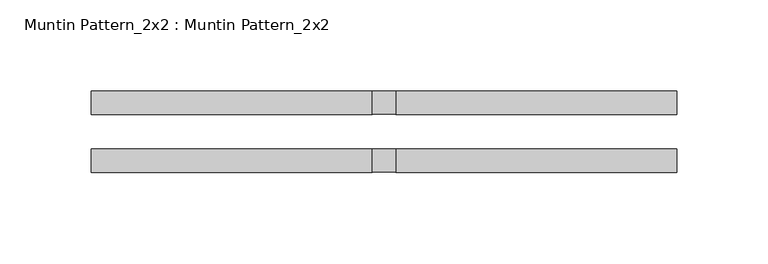
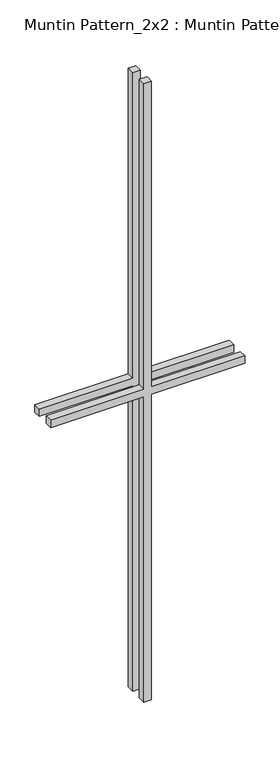
"""IFC4 building model written with IfcOpenShell, lengths in millimetres: proxy geometry, Muntin Pattern_2x2 : Muntin Pattern_2x2."""

from ifc_helpers import new_model, si_unit, frame, origin, place, context, project, spatial, polyline, outline, extrude, source, transform, mapped, element, save


def muntin_pattern_2x2_muntin_pattern_2x2_1acec82f(model_context):
    return source(origin(), model_context, "Body", "SweptSolid", [
        extrude(outline(polyline([(546.1, -6.35), (546.1, -160.3375), (533.4, -160.3375), (533.4, -6.35), (0.0, -6.35), (0.0, 6.35), (533.4, 6.35), (533.4, 160.3375), (546.1, 160.3375), (546.1, 6.35), (1079.5, 6.35), (1079.5, -6.35), (546.1, -6.35)])), frame((0.0, 9.525, 0.0), z_axis=(0.0, 1.0, 0.0), x_axis=(0.0, 0.0, 1.0)), (0.0, 0.0, 1.0), 12.7),
        extrude(outline(polyline([(546.1, -6.35), (546.1, -160.3375), (533.4, -160.3375), (533.4, -6.35), (0.0, -6.35), (0.0, 6.35), (533.4, 6.35), (533.4, 160.3375), (546.1, 160.3375), (546.1, 6.35), (1079.5, 6.35), (1079.5, -6.35), (546.1, -6.35)])), frame((0.0, -22.225, 0.0), z_axis=(0.0, 1.0, 0.0), x_axis=(0.0, 0.0, 1.0)), (0.0, 0.0, 1.0), 12.7),
    ])


if __name__ == "__main__":
    model = new_model("IFC4")
    model_context = context("Model", 3, world=origin())
    ifc_project = project(units=[si_unit("LENGTHUNIT", "METRE", prefix="MILLI")], contexts=[model_context])
    site = spatial("IfcSite", under=ifc_project)
    building = spatial("IfcBuilding", under=site)
    placement = place(None, origin())
    muntin_pattern_2x2_muntin_pattern_2x2_shape = muntin_pattern_2x2_muntin_pattern_2x2_1acec82f(model_context)
    element("IfcBuildingElementProxy", 1, Name="Muntin Pattern_2x2 : Muntin Pattern_2x2", ObjectType="Muntin Pattern_2x2 : Muntin Pattern_2x2", at=placement, inside=building, context=model_context, shape_type="MappedRepresentation", body=[
        mapped(muntin_pattern_2x2_muntin_pattern_2x2_shape, transform((0.0, 0.0, 0.0), x_axis=(1.0, 0.0, 0.0), y_axis=(0.0, 1.0, 0.0), z_axis=(0.0, 0.0, 1.0))),
    ])
    save(model, "model.ifc")

# Revit data of these elements
# Type "Muntin Pattern_2x2 : Muntin Pattern_2x2"
#   Width [instance default] = 4' - 0"
#   Thickness = 0' - 0 1/2"
#   Height [instance default] = 4' - 0"
#   Distance = 0' - 0 3/4"
#   Interior Material [instance default] = none
#   Exterior Material [instance default] = none
#   Default Elevation = 0
# Element 1 (IfcBuildingElementProxy, "Muntin Pattern_2x2 : Muntin Pattern_2x2")
#   Width = 1' - 0 5/8"
#   Height = 3' - 6 1/2"
#   Interior Material = Wood - Stained
#   Materials on its faces: "Wood - Stained"
# Materials
#   "Wood - Stained": class "Wood", colour RGB 224 178 126, transparency 0, Cost = 0
